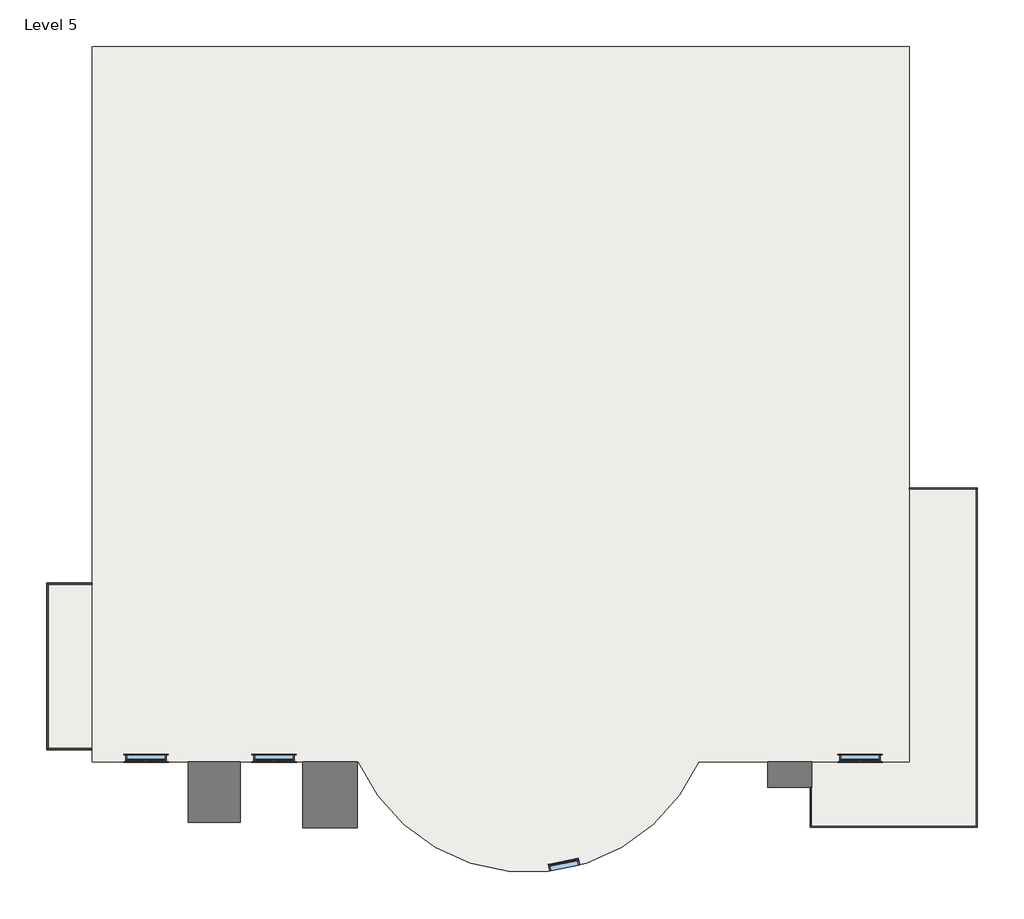
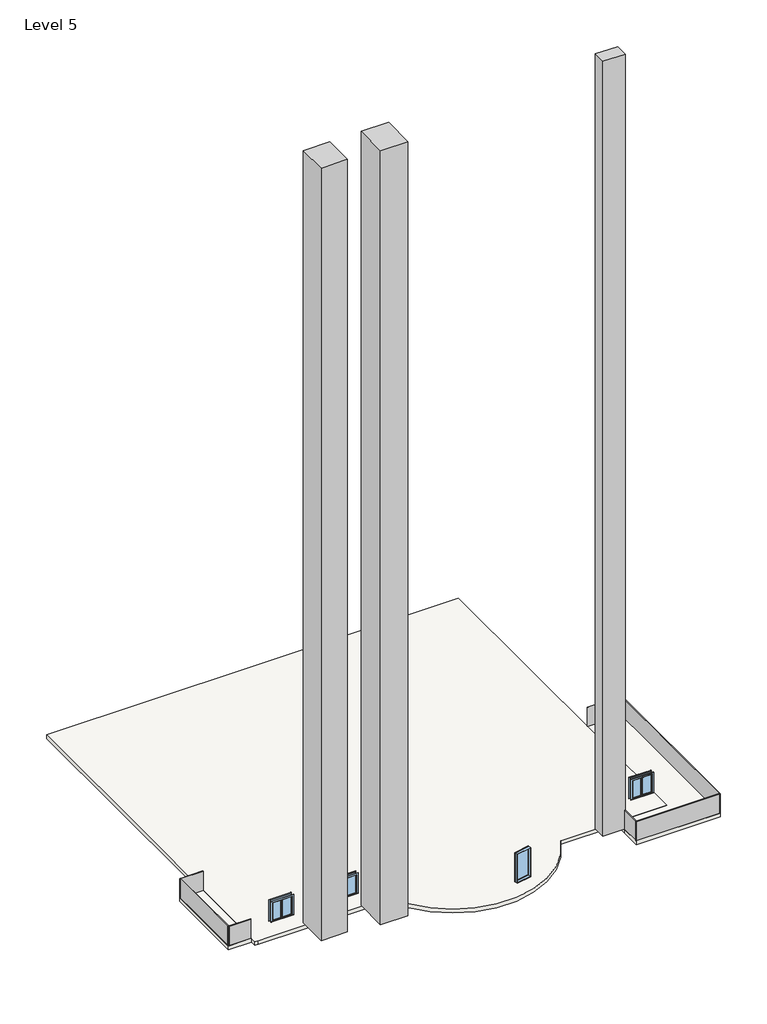
# One storey: 7 plates, 4 windows, 3 proxies, 3 slabs.
"""IFC4 building model written with IfcOpenShell, lengths in millimetres."""

from ifc_helpers import new_model, si_unit, point, frame, frame_2d, origin, place, context, project, spatial, polyline, circle_curve, trimmed, segment, composite_curve, outline, extrude, transform, mapped, element, save
from components import generic_models_1_generic_models_1_b762b88f, generic_models_2_generic_models_2_5afbfd34, generic_models_3_generic_models_3_61dd9a31, system_panel_glazed_7d767388, system_panel_glazed_246808bb, system_panel_glazed_c55d8a5b, system_panel_glazed_a5f349e9, system_panel_glazed_5a380d23, system_panel_glazed_144e3648, system_panel_glazed_8157f083, window_0862ab64, window_9a779fa2

model = new_model("IFC4")

# Units and contexts
model_context = context("Model", 3, world=origin())
ifc_project = project(units=[si_unit("LENGTHUNIT", "METRE", prefix="MILLI")], contexts=[model_context])

# Site, building, storey
site = spatial("IfcSite", under=ifc_project)
building = spatial("IfcBuilding", under=site)
storey = spatial("IfcBuildingStorey", under=building, Name="Level 5", Elevation=6553.2)

# Proxies
placement = place(None, origin())
generic_models_1_generic_models_1_shape = generic_models_1_generic_models_1_b762b88f(model_context)
element("IfcBuildingElementProxy", 1, Name="Generic Models 1 : Generic Models 1", ObjectType="Generic Models 1 : Generic Models 1", at=placement, inside=storey, context=model_context, shape_type="MappedRepresentation", body=[
    mapped(generic_models_1_generic_models_1_shape, transform((0.0, 0.0, 0.0), x_axis=(1.0, 0.0, 0.0), y_axis=(0.0, 1.0, 0.0), z_axis=(0.0, 0.0, 1.0))),
])
generic_models_2_generic_models_2_shape = generic_models_2_generic_models_2_5afbfd34(model_context)
element("IfcBuildingElementProxy", 2, Name="Generic Models 2 : Generic Models 2", ObjectType="Generic Models 2 : Generic Models 2", at=placement, inside=storey, context=model_context, shape_type="MappedRepresentation", body=[
    mapped(generic_models_2_generic_models_2_shape, transform((0.0, 0.0, 0.0), x_axis=(1.0, 0.0, 0.0), y_axis=(0.0, 1.0, 0.0), z_axis=(0.0, 0.0, 1.0))),
])
generic_models_3_generic_models_3_shape = generic_models_3_generic_models_3_61dd9a31(model_context)
element("IfcBuildingElementProxy", 3, Name="Generic Models 3 : Generic Models 3", ObjectType="Generic Models 3 : Generic Models 3", at=placement, inside=storey, context=model_context, shape_type="MappedRepresentation", body=[
    mapped(generic_models_3_generic_models_3_shape, transform((0.0, 0.0, 0.0), x_axis=(1.0, 0.0, 0.0), y_axis=(0.0, 1.0, 0.0), z_axis=(0.0, 0.0, 1.0))),
])

# Plates
system_panel_glazed_shape = system_panel_glazed_7d767388(model_context)
element("IfcPlate", 4, ObjectType="System Panel : Glazed", at=placement, inside=storey, context=model_context, shape_type="MappedRepresentation", body=[
    mapped(system_panel_glazed_shape, transform((-17306.4505427, -13719.2239591, 6553.2), x_axis=(1.0, 0.0, 0.0), y_axis=(0.0, 1.0, 0.0), z_axis=(0.0, 0.0, 1.0))),
])
system_panel_glazed_2_shape = system_panel_glazed_246808bb(model_context)
element("IfcPlate", 5, ObjectType="System Panel : Glazed", at=placement, inside=storey, context=model_context, shape_type="MappedRepresentation", body=[
    mapped(system_panel_glazed_2_shape, transform((-17293.7505427, -8690.0239591, 6553.2), x_axis=(-1.0, 0.0, 0.0), y_axis=(0.0, -1.0, 0.0), z_axis=(0.0, 0.0, 1.0))),
])
system_panel_glazed_3_shape = system_panel_glazed_c55d8a5b(model_context)
element("IfcPlate", 6, ObjectType="System Panel : Glazed", at=placement, inside=storey, context=model_context, shape_type="MappedRepresentation", body=[
    mapped(system_panel_glazed_3_shape, transform((-17979.5505427, -11204.6239591, 6553.2), x_axis=(0.0, -1.0, 0.0), y_axis=(1.0, 0.0, 0.0), z_axis=(0.0, 0.0, 1.0))),
])
system_panel_glazed_4_shape = system_panel_glazed_a5f349e9(model_context)
element("IfcPlate", 7, ObjectType="System Panel : Glazed", at=placement, inside=storey, context=model_context, shape_type="MappedRepresentation", body=[
    mapped(system_panel_glazed_4_shape, transform((7518.8744573, -16008.4808221, 6553.2), x_axis=(-1.0, 0.0, 0.0), y_axis=(0.0, -1.0, 0.0), z_axis=(0.0, 0.0, 1.0))),
])
system_panel_glazed_5_shape = system_panel_glazed_5a380d23(model_context)
element("IfcPlate", 8, ObjectType="System Panel : Glazed", at=placement, inside=storey, context=model_context, shape_type="MappedRepresentation", body=[
    mapped(system_panel_glazed_5_shape, transform((9007.9494573, -5889.2425462, 6553.2), x_axis=(1.0, 0.0, 0.0), y_axis=(0.0, 1.0, 0.0), z_axis=(0.0, 0.0, 1.0))),
])
system_panel_glazed_6_shape = system_panel_glazed_144e3648(model_context)
element("IfcPlate", 9, ObjectType="System Panel : Glazed", at=placement, inside=storey, context=model_context, shape_type="MappedRepresentation", body=[
    mapped(system_panel_glazed_6_shape, transform((9985.8494573, -10964.7366842, 6553.2), x_axis=(0.0, -1.0, 0.0), y_axis=(1.0, 0.0, 0.0), z_axis=(0.0, 0.0, 1.0))),
])
system_panel_glazed_7_shape = system_panel_glazed_8157f083(model_context)
element("IfcPlate", 10, ObjectType="System Panel : Glazed", at=placement, inside=storey, context=model_context, shape_type="MappedRepresentation", body=[
    mapped(system_panel_glazed_7_shape, transform((5058.2494573, -15455.5543258, 6553.2), x_axis=(0.0, 1.0, 0.0), y_axis=(-1.0, 0.0, 0.0), z_axis=(0.0, 0.0, 1.0))),
])

# Slabs
element("IfcSlab", 11, ObjectType="9\"", at=placement, inside=storey, context=model_context, shape_type="SweptSolid", body=[
    extrude(outline(composite_curve([segment(polyline([(-16607.9505427, 7456.0832838), (7979.2494573, 7456.0832838), (7979.2494573, -14083.1167162), (1652.8739931, -14083.1167162)]), True, "CONTINUOUS"), segment(trimmed(circle_curve(frame_2d((-3476.1505427, -11793.4009164)), 5616.9111737), [point((1652.8739931, -14083.1167162))], [point((-8605.1750786, -14083.1167162))], False, "CARTESIAN"), True, "CONTINUOUS"), segment(polyline([(-8605.1750786, -14083.1167162), (-16404.7505427, -14083.1167162), (-16607.9505427, -14083.1167162), (-16607.9505427, 7456.0832838)]), True, "CONTINUOUS")], self_intersect=False)), frame((0.0, 0.0, 6327.8754188), z_axis=(0.0, 0.0, 1.0), x_axis=(1.0, 0.0, 0.0)), (0.0, 0.0, 1.0), 228.6),
])
element("IfcSlab", 12, ObjectType="9\"", at=placement, inside=storey, context=model_context, shape_type="SweptSolid", body=[
    extrude(outline(polyline([(-17979.5505427, -8690.0239591), (-16607.9505427, -8690.0239591), (-16607.9505427, -13719.2239591), (-17979.5505427, -13719.2239591), (-17979.5505427, -8690.0239591)])), frame((0.0, 0.0, 6324.6), z_axis=(0.0, 0.0, 1.0), x_axis=(1.0, 0.0, 0.0)), (0.0, 0.0, 1.0), 228.6),
])
element("IfcSlab", 13, ObjectType="9\"", at=placement, inside=storey, context=model_context, shape_type="SweptSolid", body=[
    extrude(outline(polyline([(5007.4494573, -14840.0808221), (5007.4494573, -14078.0808221), (7191.8494573, -14078.0808221), (7395.0494573, -14078.0808221), (7395.0494573, -5848.4808221), (10036.6494573, -5848.4808221), (10036.6494573, -14840.0808221), (10036.6494573, -16059.2808221), (5007.4494573, -16059.2808221), (5007.4494573, -14840.0808221)])), frame((0.0, 0.0, 6324.6), z_axis=(0.0, 0.0, 1.0), x_axis=(1.0, 0.0, 0.0)), (0.0, 0.0, 1.0), 228.6),
])

# Windows
window_shape = window_0862ab64(model_context)
element("IfcWindow", 14, ObjectType="Casement Dbl with Trim : 48\" x 48\"", at=placement, inside=storey, context=model_context, shape_type="MappedRepresentation", body=[
    mapped(window_shape, transform((-14982.3505427, -13957.4308221, 6553.2), x_axis=(-1.0, 0.0, 0.0), y_axis=(0.0, -1.0, 0.0), z_axis=(0.0, 0.0, 1.0))),
])
element("IfcWindow", 15, ObjectType="Casement Dbl with Trim : 48\" x 48\"", at=placement, inside=storey, context=model_context, shape_type="MappedRepresentation", body=[
    mapped(window_shape, transform((-11129.6382271, -13957.4308221, 6553.2), x_axis=(-1.0, 0.0, 0.0), y_axis=(0.0, -1.0, 0.0), z_axis=(0.0, 0.0, 1.0))),
])
element("IfcWindow", 16, ObjectType="Casement Dbl with Trim : 48\" x 48\"", at=placement, inside=storey, context=model_context, shape_type="MappedRepresentation", body=[
    mapped(window_shape, transform((6506.0494573, -13957.4308221, 6742.4183808), x_axis=(-1.0, 0.0, 0.0), y_axis=(0.0, -1.0, 0.0), z_axis=(0.0, 0.0, 1.0))),
])
window_2_shape = window_9a779fa2(model_context)
element("IfcWindow", 17, ObjectType="Fixed : 36\" x 72\"", at=placement, inside=storey, context=model_context, shape_type="MappedRepresentation", body=[
    mapped(window_2_shape, transform((-2369.9451114, -17171.9936037, 7123.987617), x_axis=(0.9809073331069971, 0.19447571533977878, 0.0), y_axis=(-0.19447571533977878, 0.9809073331069971, 0.0), z_axis=(0.0, 0.0, 1.0))),
])

save(model, "model.ifc")

# Revit data of these elements
# Type "System Panel : Glazed"
#   Construction Type Id = "GSP4R"
#   Analytic Construction = "1/8 in Pilkington single glazing"
#   Visual Light Transmittance = 0.9
#   Solar Heat Gain Coefficient = 0.86
#   Heat Transfer Coefficient (U) = 1.18115 BTU/(h·ft²·°F)
# Type "9\""
#   Assembly Code = "B1010"
#   Function = 0
#   Layers, outside or top first: 0' - 9" no material (function 1)
# Type "Casement Dbl with Trim : 48\" x 48\""
#   Type Mark = "10"
#   Construction Type Id = "GSP4R"
#   Assembly Code = "B2020100"
#   Analytic Construction = "1/8 in Pilkington single glazing"
#   Visual Light Transmittance = 0.9
#   Solar Heat Gain Coefficient = 0.78
#   Heat Transfer Coefficient (U) = 0.6496 BTU/(h·ft²·°F)
#   Height = 4' - 0"
#   Default Sill Height = 3' - 0"
#   Trim Projection - Ext. = 0' - 0 1/2"
#   Trim Projection - Int. = 0' - 0 3/4"
#   Trim Width - Exterior = 0' - 3 1/2"
#   Trim Width - Interior = 0' - 3 1/2"
#   Width = 4' - 0"
#   Window Inset = 0' - 0 3/4"
#   Define Thermal Properties by = 1
#   Glass Pane Material = Glass
#   Sash Material = Sash
#   Trim Exterior Material = Trim
#   Trim Interior Material = Trim
#   Wall Closure = (empty or 0)
# Type "Fixed : 36\" x 72\""
#   Type Mark = "9"
#   Construction Type Id = "GSP4R"
#   Assembly Code = "B2020100"
#   Analytic Construction = "1/8 in Pilkington single glazing"
#   Visual Light Transmittance = 0.9
#   Solar Heat Gain Coefficient = 0.78
#   Heat Transfer Coefficient (U) = 0.6496 BTU/(h·ft²·°F)
#   Height = 6' - 0"
#   Default Sill Height = 1' - 0"
#   Width = 3' - 0"
#   Window Inset = 0' - 0 3/4"
#   Define Thermal Properties by = 1
#   Glass Pane Material = Glass
#   Sash Material = Sash
#   Wall Closure = (empty or 0)
# Element 1 (IfcBuildingElementProxy, "Generic Models 1 : Generic Models 1")
#   Phase Created = New Construction
# Element 2 (IfcBuildingElementProxy, "Generic Models 2 : Generic Models 2")
#   Phase Created = New Construction
# Element 3 (IfcBuildingElementProxy, "Generic Models 3 : Generic Models 3")
#   Phase Created = New Construction
# Elements 4, 5, 6, 7, 8, 9, 10 (IfcPlate, "System Panel : Glazed")
#   Phase Created = New Construction
#   Materials on its faces: "Glass"
# Element 11 (IfcSlab, "9\"")
#   built-in parameter 1001955 = 1.5708 (stored number, unit not read)
#   Height Offset From Level = 0' - 0.12895"
#   Phase Created = New Construction
#   Materials on its faces: "Default Floor"
# Element 12 (IfcSlab, "9\"")
#   built-in parameter 1001955 = 3.14159 (stored number, unit not read)
#   Height Offset From Level = 0' - 0"
#   Phase Created = New Construction
#   Materials on its faces: "Default Floor"
# Element 13 (IfcSlab, "9\"")
#   built-in parameter 1001955 = -1.5708 (stored number, unit not read)
#   Height Offset From Level = 0' - 0"
#   Phase Created = New Construction
#   Materials on its faces: "Default Floor"
# Element 14 (IfcWindow, "Casement Dbl with Trim : 48\" x 48\"")
#   Mark = "43"
#   Phase Created = New Construction
#   Materials on its faces: "Sash", "Trim", "Glass"
# Element 15 (IfcWindow, "Casement Dbl with Trim : 48\" x 48\"")
#   Mark = "44"
#   Phase Created = New Construction
#   Materials on its faces: "Sash", "Trim", "Glass"
# Element 16 (IfcWindow, "Casement Dbl with Trim : 48\" x 48\"")
#   Mark = "59"
#   Phase Created = New Construction
#   Materials on its faces: "Sash", "Trim", "Glass"
# Element 17 (IfcWindow, "Fixed : 36\" x 72\"")
#   Mark = "14"
#   Phase Created = New Construction
#   Materials on its faces: "Sash", "Glass"
# Materials
#   "Glass": class "Glass", colour RGB 0 128 192, transparency 0.75, Description = "Soda Lime Glass", Cost = 0
#   "Sash": class "Wood", colour RGB 224 178 126, transparency 0
#   "Trim": class "Wood", colour RGB 224 178 126, transparency 0
#   "Default Floor": colour RGB 128 128 128, transparency 0
